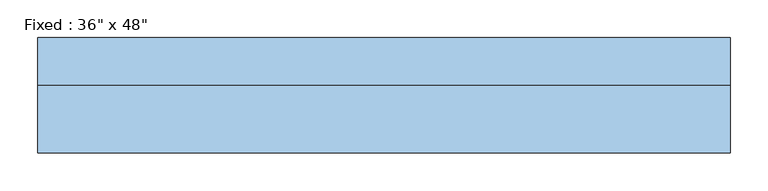
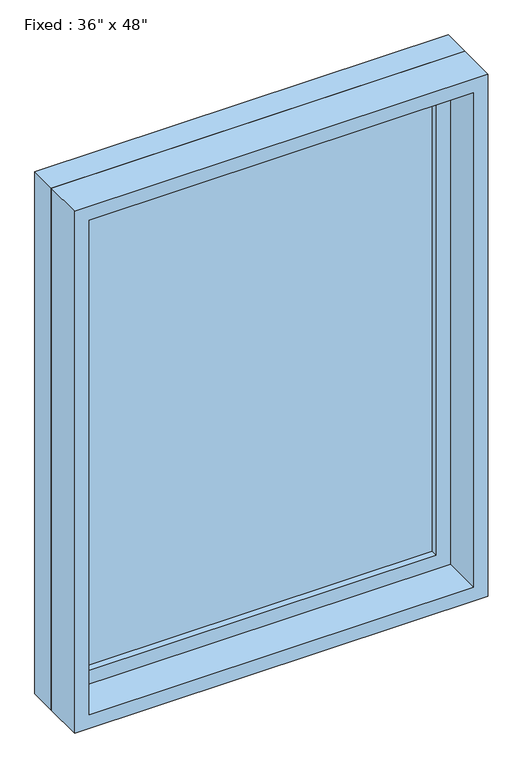
"""IFC4 building model written with IfcOpenShell, lengths in millimetres: window geometry."""

from ifc_helpers import new_model, si_unit, frame, origin, place, context, project, spatial, polyline, outline, extrude, source, transform, mapped, element, save


def window_d657a5cb(model_context):
    return source(origin(), model_context, "Body", "SweptSolid", [
        extrude(outline(polyline([(355.6, 28.575), (-431.8, 28.575), (-431.8, 41.275), (355.6, 41.275), (355.6, 28.575)])), frame((0.0, 0.0, 977.9), z_axis=(0.0, 0.0, 1.0), x_axis=(1.0, 0.0, 0.0)), (0.0, 0.0, 1.0), 1092.2),
        extrude(outline(polyline([(2114.55, -476.25), (933.45, -476.25), (933.45, 400.05), (2114.55, 400.05), (2114.55, -476.25)]), holes=[polyline([(2070.1, -431.8), (2070.1, 355.6), (977.9, 355.6), (977.9, -431.8), (2070.1, -431.8)])]), frame((0.0, 12.7, 0.0), z_axis=(0.0, 1.0, 0.0), x_axis=(0.0, 0.0, 1.0)), (0.0, 0.0, 1.0), 44.45),
        extrude(outline(polyline([(2133.6, -495.3), (914.4, -495.3), (914.4, 419.1), (2133.6, 419.1), (2133.6, -495.3)]), holes=[polyline([(2101.85, -463.55), (2101.85, 387.35), (946.15, 387.35), (946.15, -463.55), (2101.85, -463.55)])]), frame((0.0, -76.2, 0.0), z_axis=(0.0, 1.0, 0.0), x_axis=(0.0, 0.0, 1.0)), (0.0, 0.0, 1.0), 88.9),
        extrude(outline(polyline([(2133.6, 419.1), (2133.6, -495.3), (914.4, -495.3), (914.4, 419.1), (2133.6, 419.1)]), holes=[polyline([(2114.55, 400.05), (933.45, 400.05), (933.45, -476.25), (2114.55, -476.25), (2114.55, 400.05)])]), frame((0.0, 12.7, 0.0), z_axis=(0.0, 1.0, 0.0), x_axis=(0.0, 0.0, 1.0)), (0.0, 0.0, 1.0), 63.5),
    ])


if __name__ == "__main__":
    model = new_model("IFC4")
    model_context = context("Model", 3, world=origin())
    ifc_project = project(units=[si_unit("LENGTHUNIT", "METRE", prefix="MILLI")], contexts=[model_context])
    site = spatial("IfcSite", under=ifc_project)
    building = spatial("IfcBuilding", under=site)
    placement = place(None, origin())
    window_shape = window_d657a5cb(model_context)
    element("IfcWindow", 1, ObjectType="Fixed : 36\" x 48\"", at=placement, inside=building, context=model_context, shape_type="MappedRepresentation", body=[
        mapped(window_shape, transform((0.0, 0.0, 0.0), x_axis=(1.0, 0.0, 0.0), y_axis=(0.0, 1.0, 0.0), z_axis=(0.0, 0.0, 1.0))),
    ])
    save(model, "model.ifc")

# Revit data of these elements
# Type "Fixed : 36\" x 48\""
#   Type Mark = "1"
#   Construction Type Id = "GSP4R"
#   Assembly Code = "B2020100"
#   Analytic Construction = "1/8 in Pilkington single glazing"
#   Visual Light Transmittance = 0.9
#   Solar Heat Gain Coefficient = 0.78
#   Heat Transfer Coefficient (U) = 0.6496 BTU/(h·ft²·°F)
#   Height = 4' - 0"
#   Default Sill Height = 3' - 0"
#   Width = 3' - 0"
#   Window Inset = 0' - 0 3/4"
#   Define Thermal Properties by = 1
#   Define Thermal Properties by = 1
#   Glass Pane Material = Glass
#   Sash Material = Sash
#   Wall Closure = (empty or 0)
# Element 1 (IfcWindow, "Fixed : 36\" x 48\"")
#   Materials on its faces: "Sash", "Glass"
# Materials
#   "Glass": class "Glass", colour RGB 0 128 192, transparency 0.75, Description = "Soda Lime Glass", Cost = 0
#   "Sash": class "Wood", colour RGB 224 178 126, transparency 0, Cost = 0
